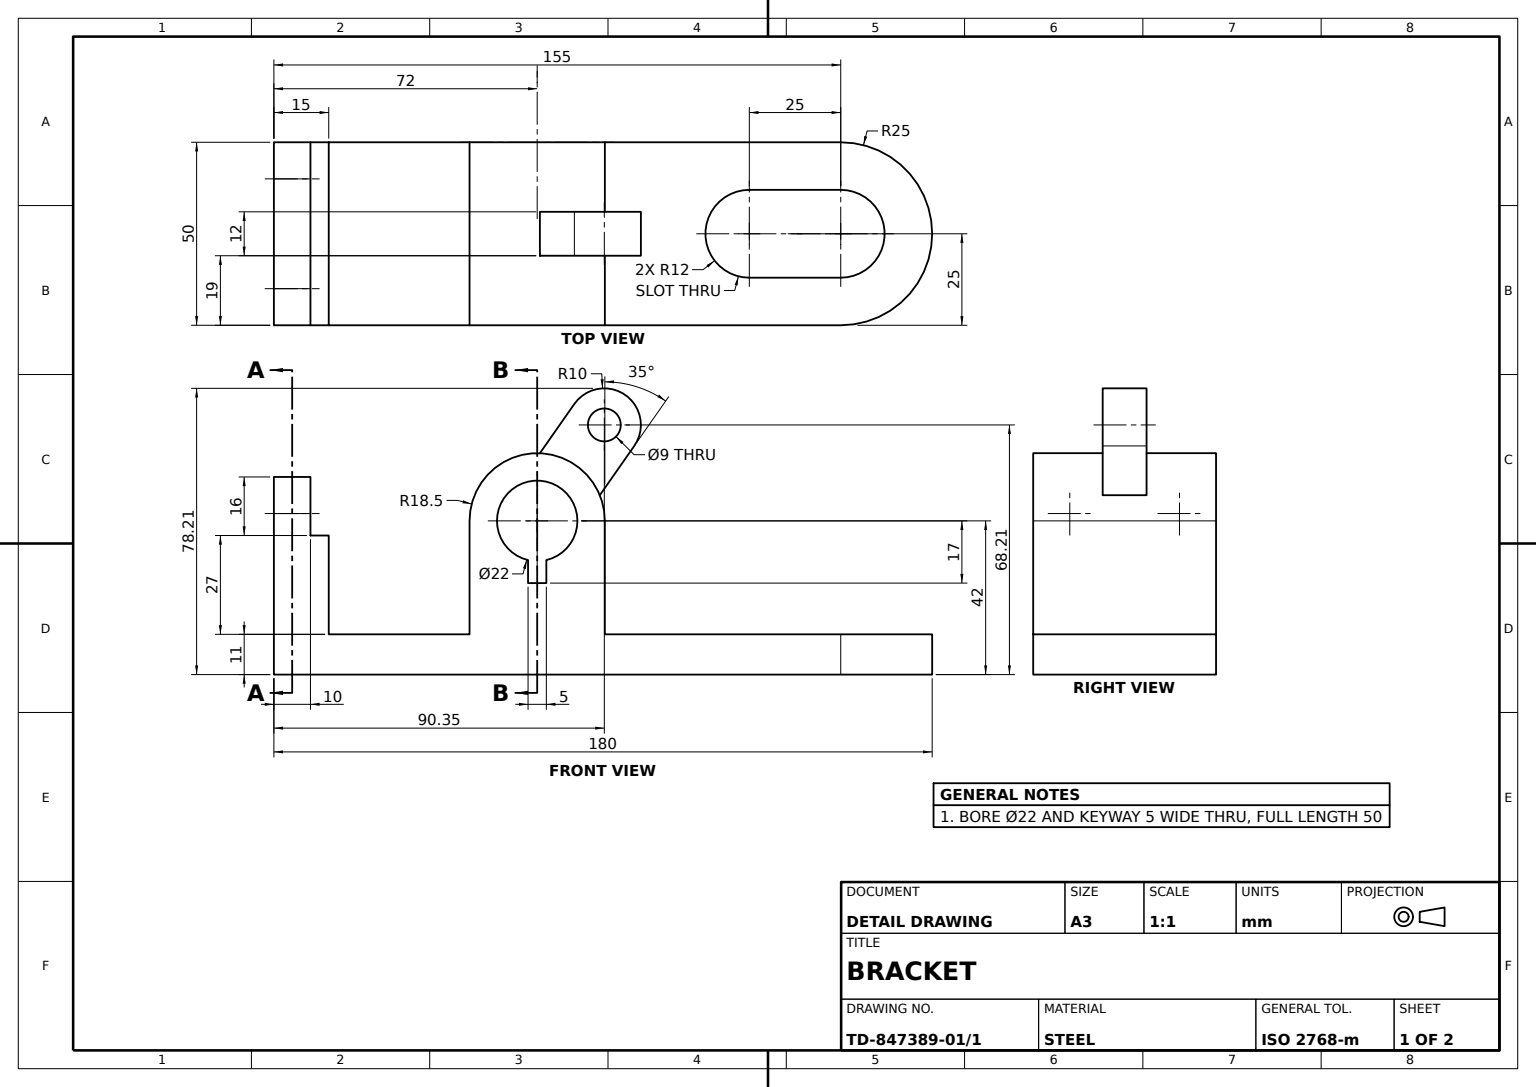
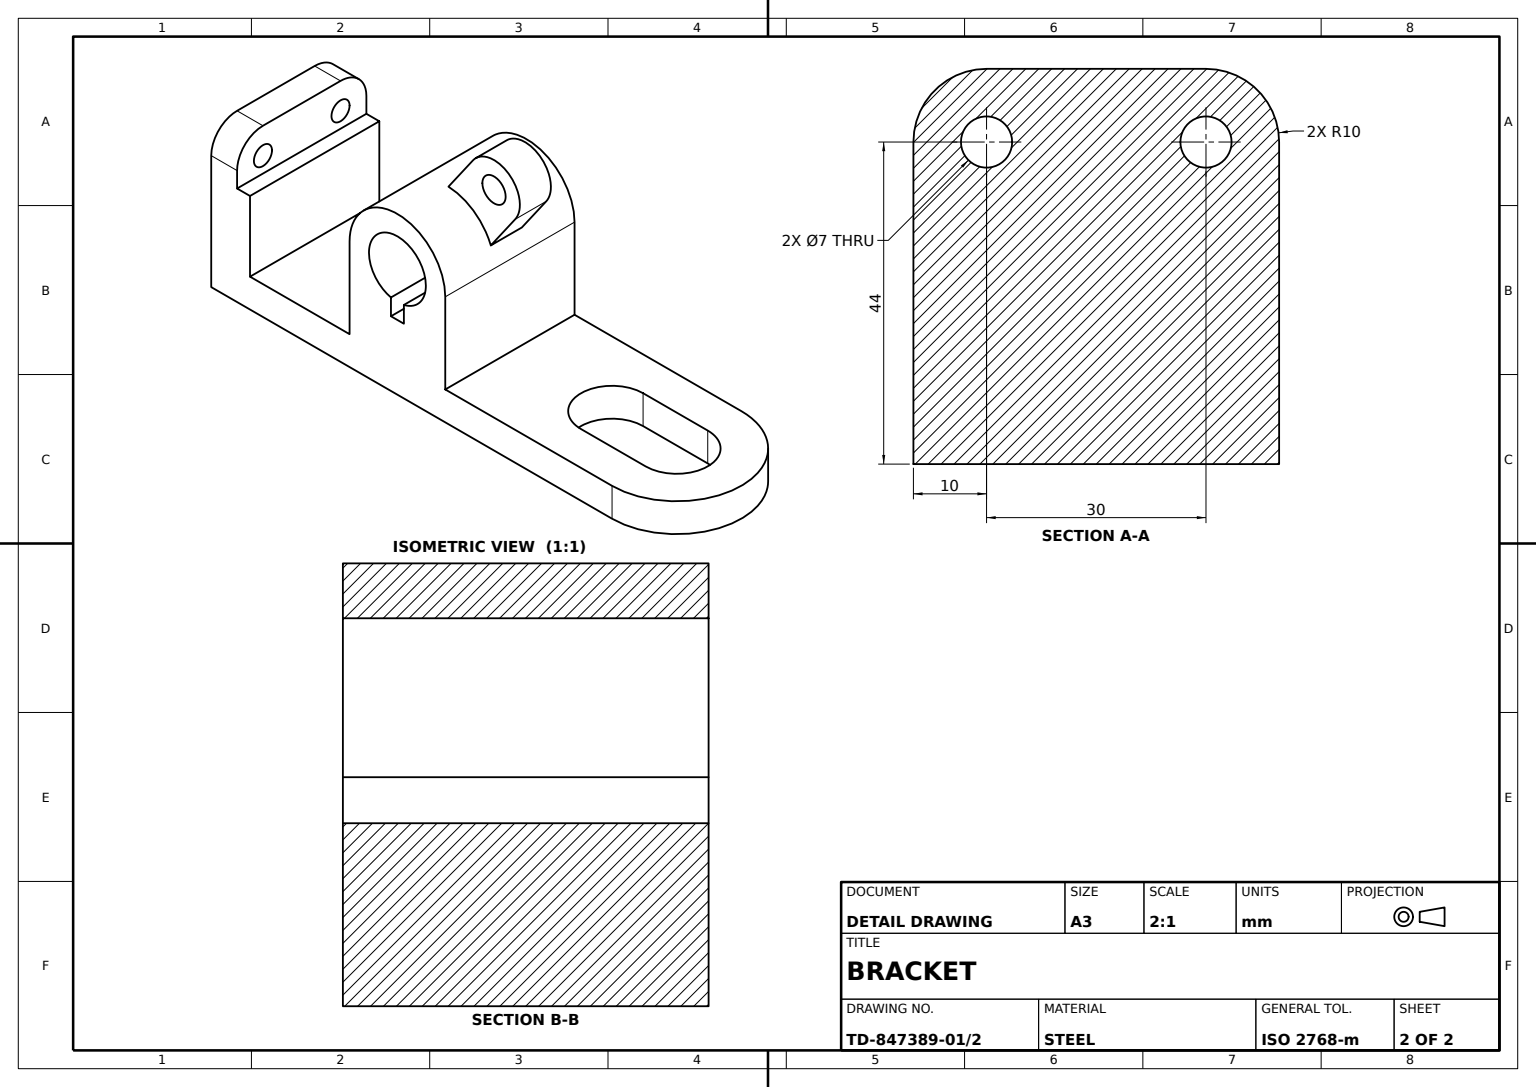
SolidWorks part; units mm, degrees
material "Plain Carbon Steel"
ref_plane "Front Plane" through (0, 0, 0) normal (0, 0, 1) x (1, 0, 0)
ref_plane "Top Plane" through (0, 0, 0) normal (0, 1, 0) x (1, 0, 0)
ref_plane "Right Plane" through (0, 0, 0) normal (1, 0, 0) x (0, 0, -1)
sketch "Base Plate Sketch" plane through (0, 0, 0) normal (0, 1, 0) x (1, 0, 0)
  line L1 (77.5, -25) -> (-77.5, -25)
  line L2 (-77.5, -25) -> (-77.5, 25)
  line L3 (-77.5, 25) -> (77.5, 25)
  arc A0 (77.5, -25) -> (77.5, 25) centre (77.5, 0) ccw
  dimension "D1" = 25
  dimension "D2" = 155
  dimension "D3" = 77.5
extrude "Base Plate 11mm" add sketch "Base Plate Sketch" along normal blind 11
sketch "Channel Cut Sketch" plane through (0, 11, 0) normal (0, 1, 0) x (1, 0, 0)
  line L1 (52.5, 12) -> (77.5, 12)
  line L2 (52.5, -12) -> (77.5, -12)
  arc A1 (77.5, -12) -> (77.5, 12) centre (77.5, 0) ccw
  arc A2 (52.5, 12) -> (52.5, -12) centre (52.5, 0) ccw
  dimension "D1" = 12
  dimension "D2" = 25
extrude "Channel Cut 12x25" cut sketch "Channel Cut Sketch" against normal blind 102
sketch "Bore Block Sketch" plane through (0, 0, 25) normal (0, 0, 1) x (1, 0, 0)
  line L2 (-24, 11) -> (13, 11)
  line L3 (13, 42) -> (13, 11)
  line L4 (-77.5, 11) -> (77.5, 11) construction
  line L6 (-24, 11) -> (-24, 42)
  arc A0 (13, 42) -> (-24, 42) centre (-5.5, 42) ccw
  dimension "D1" = 18.5
  dimension "D2" = 42
  dimension "D3" = 5.5
extrude "Bore Block" add sketch "Bore Block Sketch" against normal blind 50
sketch "Keyed Bore Sketch" plane through (0, 0, 25) normal (0, 0, 1) x (1, 0, 0)
  line L1 (-5.5, 25) -> (-3, 25)
  line L2 (-3, 25) -> (-3, 31.2879)
  line L3 (-5.5, 25) -> (-8, 25)
  line L4 (-8, 25) -> (-8, 31.2879)
  arc A0 (-3, 31.2879) -> (-8, 31.2879) centre (-5.5, 42) ccw
  dimension "D1" = 11
  dimension "D2" = 6.2879
  dimension "D3" = 5
  dimension "D4" = 6.2879
  dimension "D5" = 17
extrude "Keyed Bore Ø11" cut sketch "Keyed Bore Sketch" against normal blind 68
sketch "Angled Lug Sketch" plane through (0, 0, 0) normal (0, 0, 1) x (1, 0, 0)
  line L1 (11.6189, 49.0138) -> (21.046, 62.4771)
  line L2 (-4.7642, 60.4854) -> (4.6629, 73.9486)
  arc A0 (21.046, 62.4771) -> (4.6629, 73.9486) centre (12.8544, 68.2129) ccw
  arc A1 (11.6189, 49.0138) -> (-4.7642, 60.4854) centre (-5.5, 42) ccw
  dimension "D1" = 10
  dimension "D4" = 18.5
  dimension "D2" = 68.2129
  dimension "D3" = 12.8544
  dimension "D5" = 16.4356
  dimension "D6" = 20
  dimension "D7" = 13.4633
extrude "Angled Lug" add sketch "Angled Lug Sketch" along normal mid plane 12
sketch "Lug Hole Sketch" plane through (0, 0, 6) normal (0, 0, 1) x (1, 0, 0)
  circle A0 centre (12.8544, 68.2129) radius 4.5
  dimension "D1" = 9
extrude "Lug Hole Ø9" cut sketch "Lug Hole Sketch" against normal blind 20
sketch "End Lug Sketch" plane through (0, 11, 0) normal (0, 1, 0) x (1, 0, 0)
  line L0 (-77.5, -25) -> (-62.5, -25)
  line L1 (-77.5, -25) -> (-24, -25) construction
  line L2 (-62.5, -25) -> (-62.5, 25)
  line L3 (-24, 25) -> (-77.5, 25) construction
  line L4 (-62.5, 25) -> (-77.5, 25)
  line L5 (-77.5, 25) -> (-77.5, -25)
  dimension "D1" = 15
extrude "End Lug" add sketch "End Lug Sketch" along normal blind 27
sketch "End Lug Tip Sketch" plane through (0, 38, 0) normal (0, 1, 0) x (1, 0, 0)
  line L0 (-77.5, -25) -> (-67.5, -25)
  line L1 (-77.5, -25) -> (-62.5, -25) construction
  line L2 (-67.5, -25) -> (-67.5, 25)
  line L3 (-62.5, 25) -> (-77.5, 25) construction
  line L4 (-67.5, 25) -> (-77.5, 25)
  line L5 (-77.5, 25) -> (-77.5, -25)
  dimension "D1" = 10
extrude "End Lug Tip" add sketch "End Lug Tip Sketch" along normal blind 16
fillet "End Lug Round R10 A" radius 10 1 edges at (-72.5, 54, 25)
fillet "End Lug Round R10 B" radius 10 1 edges at (-72.5, 54, -25)
sketch "End Lug Cut Sketch" plane through (-77.5, 0, 0) normal (-1, 0, 0) x (0, 0, 1)
  circle A0 centre (15, 44) radius 3.5
  circle A1 centre (-15, 44) radius 3.5
  dimension "D1" = 7
  dimension "D2" = 7
extrude "End Lug Cut Ø7" cut sketch "End Lug Cut Sketch" against normal blind 16
